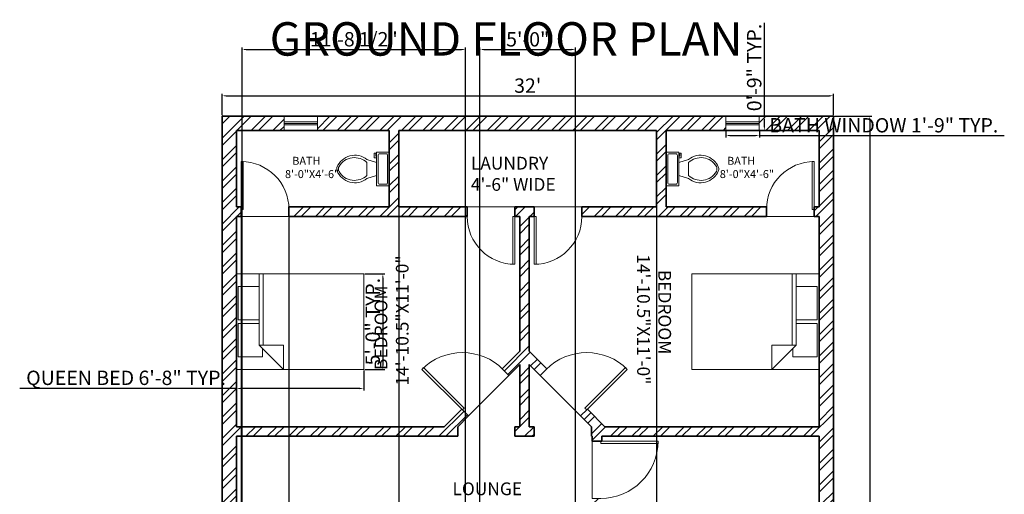
# Model space of a CAD drawing. Units: inches. Extents: x 287 to 905, y 1151 to 2037.
# Tile 5 of 5: x 287 to 905, y 1739 to 2037. Entities that reach past the tile are written whole.
import ezdxf

# ---------------------------------------------------------------- set-up
doc = ezdxf.new("R2010")
doc.units = ezdxf.units.IN
for name, color, linetype, lineweight in [('A-ANNO-DIMS', 2, 'Continuous', 18), ('A-ANNO-TEXT', 7, 'Continuous', 25), ('A-AREA-IDEN', 7, 'Continuous', 18), ('A-DOOR', 4, 'Continuous', 18), ('A-FLOR-FIXT', 8, 'Continuous', 18), ('A-FURN', 9, 'Continuous', 18), ('A-WALL', 7, 'Continuous', 35), ('A-WALL-PATT', 252, 'Continuous', 13)]:
    doc.layers.add(name, color=color, linetype=linetype, lineweight=lineweight)
doc.layers.add('A-GLAZ', color=244, linetype='Continuous', lineweight=18, true_color=0x991b1e)
doc.styles.get("Standard").update_dxf_attribs({"font": 'arial.ttf'})
doc.dimstyles.new('ISO-25', dxfattribs={"dimtxt": 9, "dimasz": 2.5, "dimexe": 1.25, "dimexo": 0.625, "dimtad": 1, "dimlunit": 3, "dimtxsty": 'Standard', "dimcen": 2.5, "dimadec": 0, "dimazin": 0, "dimtfac": 1, "dimtmove": 0, "dimatfit": 3, "dimfxl": 1, "dimarcsym": 0})

# ---------------------------------------------------------------- blocks, each defined once
blk = doc.blocks.new('*U3')
for p, q in [((0, 0), (0, -6)), ((-40, 0), (-40, -6))]:
    blk.add_line(p, q)
blk.add_lwpolyline([(0, 0), (0, 40), (-1.75, 40), (-1.75, 0)], close=True)
blk.add_arc((0, 0), 40, 90, 180)
blk = doc.blocks.new('*U2')
for p, q in [((0, 0), (0, -6)), ((40, 0), (40, -6))]:
    blk.add_line(p, q)
blk.add_lwpolyline([(0, 0), (0, 40), (1.75, 40), (1.75, 0)], close=True)
blk.add_arc((0, 0), 40, 0, 90)
blk = doc.blocks.new('*U5')
for p, q in [((-40, 0), (-40, 6)), ((0, 0), (0, 6))]:
    blk.add_line(p, q)
blk.add_lwpolyline([(0, 0), (0, -40), (-1.75, -40), (-1.75, 0)], close=True)
blk.add_arc((0, 0), 40, 180, 270)
blk = doc.blocks.new('*U4')
for p, q in [((0, 0), (0, 6)), ((40, 0), (40, 6))]:
    blk.add_line(p, q)
blk.add_lwpolyline([(0, 0), (0, -40), (1.75, -40), (1.75, 0)], close=True)
blk.add_arc((0, 0), 40, 270, 0)
blk = doc.blocks.new('*U6')
for p, q in [((0, 0), (0, -6)), ((40, 0), (40, -6))]:
    blk.add_line(p, q)
blk.add_lwpolyline([(0, 0), (0, 40), (1.75, 40), (1.75, 0)], close=True)
blk.add_arc((0, 0), 40, 0, 90)
blk = doc.blocks.new('Bed - Queen')
for p, q in [((0, -80.00003), (0, 0)), ((0, 0), (59.99999, 0)), ((59.99999, 0), (59.99999, -80.00003)), ((7.99999, -1.2), (28.79998, -1.2)), ((7.99999, -14.4), (7.99999, -1.2)), ((28.79998, -1.2), (28.79998, -14.4)), ((31.19999, -1.2), (51.99999, -1.2)), ((31.19999, -14.4), (31.19999, -1.2)), ((51.99999, -1.2), (51.99999, -16.4)), ((0, -14.4), (44.8, -14.4)), ((44.8, -16.8), (0, -16.8)), ((59.99999, -29.6), (44.8, -14.4)), ((44.8, -14.4), (44.8, -29.6)), ((51.99999, -16.4), (46.79936, -16.4)), ((44.8, -29.6), (59.99999, -29.6)), ((59.99999, -80.00003), (0, -80.00003))]:
    blk.add_line(p, q)
blk = doc.blocks.new('*U12')
for p, q in [((9.5, -6), (9.5, -2)), ((-10, -8.5), (-8, -8.5)), ((-10, -9.5), (-10, -8.5)), ((-7, -9.5), (-10, -9.5)), ((-8, -8.5), (-8, -8)), ((-7, -8), (-7, -9.5)), ((-4, -8), (-6, -14)), ((4, -8), (6, -14)), ((4, -14), (-4, -14))]:
    blk.add_line(p, q)
blk.add_lwpolyline([(10.5, -8), (10.5, 0), (-10.5, 0), (-10.5, -8)], close=True)
for points in [[(-9.5, -2), (-9.5, -6)], [(8.5, -1), (-8.5, -1)], [(-8.5, -7), (8.5, -7)]]:
    blk.add_lwpolyline(points)
for centre, radius, start, end in [((-8.62, -1.88), 0.884, 81.8699, 188.1301), ((-8.62, -6.12), 0.884, 171.8699, 278.1301), ((8.62, -1.88), 0.884, 351.8699, 98.1301), ((8.62, -6.12), 0.884, 261.8699, 8.1301), ((3.52, -21.58), 12.17, 141.46911, 247.97143), ((4.2, -21.82), 11.33, 136.36773, 238.94682), ((-3.52, -21.58), 12.17, 292.02843, 38.53071), ((-4.2, -21.82), 11.33, 301.05301, 43.63209), ((0, -27.88), 4, 245.73182, 294.26817), ((0, -29), 4, 254.86053, 285.13947)]:
    blk.add_arc(centre, radius, start, end)
blk = doc.blocks.new('*D13')
at = {"layer": 'A-ANNO-DIMS', "color": 0, "lineweight": -2, "transparency": 16777216}
for p, q in [((413.86, 1977.46), (413.86, 1990.88)), ((416.36, 1989.63), (795.36, 1989.63)), ((797.86, 1977.46), (797.86, 1990.88))]:
    blk.add_line(p, q, dxfattribs=at)
at = {"layer": 'A-ANNO-DIMS', "color": 0, "transparency": 16777216}
for points in [[(416.36, 1990.05), (416.36, 1989.22), (413.86, 1989.63)], [(795.36, 1990.05), (795.36, 1989.22), (797.86, 1989.63)]]:
    blk.add_solid(points, dxfattribs=at)
at = {"layer": 'Defpoints', "color": 0, "transparency": 16777216}
for p in [(797.86, 1989.63), (413.86, 1976.83), (797.86, 1976.83)]:
    blk.add_point(p, dxfattribs=at)
at = {"layer": 'A-ANNO-DIMS', "color": 0, "transparency": 16777216, "insert": (605.86, 1994.86), "char_height": 9, "attachment_point": 5}
blk.add_mtext("32'", dxfattribs=at)
blk = doc.blocks.new('*D14')
at = {"layer": 'A-ANNO-DIMS', "color": 0, "lineweight": -2, "transparency": 16777216}
for p, q in [((798.48, 1976.83), (822.01, 1976.83)), ((820.76, 1974.33), (820.76, 1280.33)), ((798.48, 1277.83), (822.01, 1277.83))]:
    blk.add_line(p, q, dxfattribs=at)
at = {"layer": 'A-ANNO-DIMS', "color": 0, "transparency": 16777216}
for points in [[(820.35, 1974.33), (821.18, 1974.33), (820.76, 1976.83)], [(820.35, 1280.33), (821.18, 1280.33), (820.76, 1277.83)]]:
    blk.add_solid(points, dxfattribs=at)
at = {"layer": 'Defpoints', "color": 0, "transparency": 16777216}
for p in [(797.86, 1976.83), (797.86, 1277.83), (820.76, 1277.83)]:
    blk.add_point(p, dxfattribs=at)
at = {"layer": 'A-ANNO-DIMS', "color": 0, "transparency": 16777216, "insert": (815.54, 1627.33), "char_height": 9, "attachment_point": 5, "rotation": 90}
blk.add_mtext('58\'-3"', dxfattribs=at)
blk = doc.blocks.new('WIN-21IN')
for p, q in [((-10.5, 1), (10.5, 1)), ((-10.5, 0), (10.5, 0)), ((-10.5, -1), (10.5, -1))]:
    blk.add_line(p, q)
blk.add_lwpolyline([(-10.5, 4.5), (10.5, 4.5), (10.5, -4.5), (-10.5, -4.5)], close=True)
blk = doc.blocks.new('*D18')
at = {"layer": 'A-ANNO-DIMS', "color": 0, "lineweight": -2, "transparency": 16777216}
for p, q in [((422.86, 1817.21), (422.86, 1804.58)), ((502.86, 1817.21), (502.86, 1804.58)), ((422.86, 1805.83), (286.72, 1805.83)), ((500.36, 1805.83), (425.36, 1805.83))]:
    blk.add_line(p, q, dxfattribs=at)
at = {"layer": 'A-ANNO-DIMS', "color": 0, "transparency": 16777216}
for points in [[(425.36, 1806.25), (425.36, 1805.42), (422.86, 1805.83)], [(500.36, 1806.25), (500.36, 1805.42), (502.86, 1805.83)]]:
    blk.add_solid(points, dxfattribs=at)
at = {"layer": 'Defpoints', "color": 0, "transparency": 16777216}
for p in [(422.86, 1817.83), (502.86, 1817.83), (422.86, 1805.83)]:
    blk.add_point(p, dxfattribs=at)
at = {"layer": 'A-ANNO-DIMS', "color": 0, "transparency": 16777216, "insert": (353.54, 1811.39), "char_height": 9, "attachment_point": 5}
blk.add_mtext('QUEEN BED 6\'-8" TYP.', dxfattribs=at)
blk = doc.blocks.new('*D19')
at = {"layer": 'A-ANNO-DIMS', "color": 0, "lineweight": -2, "transparency": 16777216}
for p, q in [((503.48, 1877.83), (516.11, 1877.83)), ((514.86, 1875.33), (514.86, 1820.33)), ((503.48, 1817.83), (516.11, 1817.83))]:
    blk.add_line(p, q, dxfattribs=at)
at = {"layer": 'A-ANNO-DIMS', "color": 0, "transparency": 16777216}
for points in [[(514.44, 1875.33), (515.27, 1875.33), (514.86, 1877.83)], [(514.44, 1820.33), (515.27, 1820.33), (514.86, 1817.83)]]:
    blk.add_solid(points, dxfattribs=at)
at = {"layer": 'Defpoints', "color": 0, "transparency": 16777216}
for p in [(502.86, 1877.83), (502.86, 1817.83), (514.86, 1817.83)]:
    blk.add_point(p, dxfattribs=at)
at = {"layer": 'A-ANNO-DIMS', "color": 0, "transparency": 16777216, "insert": (509.64, 1847.83), "char_height": 9, "attachment_point": 5, "rotation": 90}
blk.add_mtext('5\'-0" TYP.', dxfattribs=at)
blk = doc.blocks.new('*D20')
at = {"layer": 'A-ANNO-DIMS', "color": 0, "lineweight": -2, "transparency": 16777216}
for p, q in [((730.36, 1967.21), (730.36, 1963.43)), ((751.36, 1967.21), (751.36, 1963.43)), ((732.86, 1964.68), (748.86, 1964.68)), ((751.36, 1964.68), (905.25, 1964.68))]:
    blk.add_line(p, q, dxfattribs=at)
at = {"layer": 'A-ANNO-DIMS', "color": 0, "transparency": 16777216}
for points in [[(732.86, 1965.1), (732.86, 1964.27), (730.36, 1964.68)], [(748.86, 1965.1), (748.86, 1964.27), (751.36, 1964.68)]]:
    blk.add_solid(points, dxfattribs=at)
at = {"layer": 'Defpoints', "color": 0, "transparency": 16777216}
for p in [(730.36, 1967.83), (751.36, 1967.83), (751.36, 1964.68)]:
    blk.add_point(p, dxfattribs=at)
at = {"layer": 'A-ANNO-DIMS', "color": 0, "transparency": 16777216, "insert": (829.55, 1969.96), "char_height": 9, "attachment_point": 5}
blk.add_mtext('BATH WINDOW 1\'-9" TYP.', dxfattribs=at)
blk = doc.blocks.new('*D21')
at = {"layer": 'A-ANNO-DIMS', "color": 0, "lineweight": -2, "transparency": 16777216}
for p, q in [((754.51, 1976.83), (754.51, 2035.44)), ((751.98, 1976.83), (755.76, 1976.83)), ((754.51, 1970.33), (754.51, 1974.33)), ((751.98, 1967.83), (755.76, 1967.83))]:
    blk.add_line(p, q, dxfattribs=at)
at = {"layer": 'A-ANNO-DIMS', "color": 0, "transparency": 16777216}
for points in [[(754.09, 1974.33), (754.92, 1974.33), (754.51, 1976.83)], [(754.09, 1970.33), (754.92, 1970.33), (754.51, 1967.83)]]:
    blk.add_solid(points, dxfattribs=at)
at = {"layer": 'Defpoints', "color": 0, "transparency": 16777216}
for p in [(751.36, 1976.83), (754.51, 1976.83), (751.36, 1967.83)]:
    blk.add_point(p, dxfattribs=at)
at = {"layer": 'A-ANNO-DIMS', "color": 0, "transparency": 16777216, "insert": (749.29, 2007.39), "char_height": 9, "attachment_point": 5, "rotation": 90}
blk.add_mtext('0\'-9" TYP.', dxfattribs=at)
blk = doc.blocks.new('*D32')
at = {"layer": 'A-ANNO-DIMS', "color": 0, "lineweight": -2, "transparency": 16777216}
for p, q in [((426.39, 1284.46), (426.39, 2019.96)), ((428.89, 2018.71), (564.36, 2018.71)), ((566.86, 1284.46), (566.86, 2019.96))]:
    blk.add_line(p, q, dxfattribs=at)
at = {"layer": 'A-ANNO-DIMS', "color": 0, "transparency": 16777216}
for points in [[(428.89, 2019.12), (428.89, 2018.29), (426.39, 2018.71)], [(564.36, 2019.12), (564.36, 2018.29), (566.86, 2018.71)]]:
    blk.add_solid(points, dxfattribs=at)
at = {"layer": 'Defpoints', "color": 0, "transparency": 16777216}
for p in [(566.86, 2018.71), (426.39, 1283.83), (566.86, 1283.83)]:
    blk.add_point(p, dxfattribs=at)
at = {"layer": 'A-ANNO-DIMS', "color": 0, "transparency": 16777216, "insert": (496.62, 2023.99), "char_height": 9, "attachment_point": 5}
blk.add_mtext('11\'-8 1/2"', dxfattribs=at)
blk = doc.blocks.new('*D33')
at = {"layer": 'A-ANNO-DIMS', "color": 0, "lineweight": -2, "transparency": 16777216}
for p, q in [((575.86, 1284.46), (575.86, 2019.96)), ((578.36, 2018.71), (633.36, 2018.71)), ((635.86, 1284.46), (635.86, 2019.96))]:
    blk.add_line(p, q, dxfattribs=at)
at = {"layer": 'A-ANNO-DIMS', "color": 0, "transparency": 16777216}
for points in [[(578.36, 2019.12), (578.36, 2018.29), (575.86, 2018.71)], [(633.36, 2019.12), (633.36, 2018.29), (635.86, 2018.71)]]:
    blk.add_solid(points, dxfattribs=at)
at = {"layer": 'Defpoints', "color": 0, "transparency": 16777216}
for p in [(635.86, 2018.71), (575.86, 1283.83), (635.86, 1283.83)]:
    blk.add_point(p, dxfattribs=at)
at = {"layer": 'A-ANNO-DIMS', "color": 0, "transparency": 16777216, "insert": (605.86, 2023.93), "char_height": 9, "attachment_point": 5}
blk.add_mtext('5\'-0"', dxfattribs=at)
blk = doc.blocks.new('*D37')
at = {"layer": 'A-ANNO-DIMS', "color": 0, "lineweight": -2, "transparency": 16777216}
for p, q in [((524.86, 1967.21), (524.86, 1157.65)), ((686.86, 1967.21), (686.86, 1157.65)), ((527.36, 1158.9), (684.36, 1158.9))]:
    blk.add_line(p, q, dxfattribs=at)
at = {"layer": 'A-ANNO-DIMS', "color": 0, "transparency": 16777216}
for points in [[(527.36, 1159.32), (527.36, 1158.49), (524.86, 1158.9)], [(684.36, 1159.32), (684.36, 1158.49), (686.86, 1158.9)]]:
    blk.add_solid(points, dxfattribs=at)
at = {"layer": 'Defpoints', "color": 0, "transparency": 16777216}
for p in [(524.86, 1967.83), (686.86, 1967.83), (686.86, 1158.9)]:
    blk.add_point(p, dxfattribs=at)
at = {"layer": 'A-ANNO-DIMS', "color": 0, "transparency": 16777216, "insert": (605.86, 1164.13), "char_height": 9, "attachment_point": 5}
blk.add_mtext('13\'-6"', dxfattribs=at)
blk = doc.blocks.new('*D38')
at = {"layer": 'A-ANNO-DIMS', "color": 0, "lineweight": -2, "transparency": 16777216}
for p, q in [((425.86, 1913.21), (425.86, 1157.65)), ((455.86, 1913.21), (455.86, 1157.65)), ((428.36, 1158.9), (453.36, 1158.9))]:
    blk.add_line(p, q, dxfattribs=at)
at = {"layer": 'A-ANNO-DIMS', "color": 0, "transparency": 16777216}
for points in [[(428.36, 1159.32), (428.36, 1158.49), (425.86, 1158.9)], [(453.36, 1159.32), (453.36, 1158.49), (455.86, 1158.9)]]:
    blk.add_solid(points, dxfattribs=at)
at = {"layer": 'Defpoints', "color": 0, "transparency": 16777216}
for p in [(425.86, 1913.83), (455.86, 1913.83), (455.86, 1158.9)]:
    blk.add_point(p, dxfattribs=at)
at = {"layer": 'A-ANNO-DIMS', "color": 0, "transparency": 16777216, "insert": (440.86, 1164.12), "char_height": 9, "attachment_point": 5}
blk.add_mtext('2\'-6"', dxfattribs=at)

msp = doc.modelspace()

# ---------------------------------------------------------------- hatches: boundary and pattern name
at = {"layer": 'A-WALL-PATT'}
h = msp.add_hatch(dxfattribs=at)
h.set_pattern_fill('ANSI32', color=256)
h.paths.add_polyline_path([(422.857, 1775.833), (561.857, 1775.833), (561.857, 1781.833), (568.629, 1788.605), (564.387, 1792.848), (553.372, 1781.833), (422.857, 1781.833), (422.857, 1913.833), (425.857, 1913.833), (425.857, 1919.833), (422.857, 1919.833), (422.857, 1967.833), (452.78, 1967.833), (452.78, 1976.833), (413.857, 1976.833), (413.857, 1502.833), (436.063, 1502.833), (436.063, 1511.833), (422.857, 1511.833), (422.857, 1625.833), (474.857, 1625.833), (474.857, 1631.833), (422.857, 1631.833)])
h = msp.add_hatch(dxfattribs=at)
h.set_pattern_fill('ANSI32', color=256)
h.paths.add_polyline_path([(604.357, 1511.833), (519.857, 1511.833), (519.857, 1625.833), (607.357, 1625.833), (607.357, 1631.833), (510.857, 1631.833), (510.857, 1625.833), (513.857, 1625.833), (513.857, 1511.833), (496.063, 1511.833), (496.063, 1502.833), (604.357, 1502.833)])
h.paths.add_polyline_path([(652.357, 1511.833), (652.357, 1514.833), (643.357, 1514.833), (643.357, 1511.833), (640.357, 1511.833), (640.357, 1505.833), (643.357, 1505.833), (643.357, 1370.833), (690.607, 1370.833), (690.607, 1379.833), (652.357, 1379.833)])
h.paths.add_polyline_path([(797.857, 1582.055), (788.857, 1582.055), (788.857, 1571.833), (703.357, 1571.833), (703.357, 1574.833), (697.357, 1574.833), (697.357, 1571.833), (652.357, 1571.833), (652.357, 1574.833), (646.357, 1574.833), (646.357, 1562.833), (652.357, 1562.833), (652.357, 1565.833), (788.857, 1565.833), (788.857, 1379.833), (750.607, 1379.833), (750.607, 1370.833), (797.857, 1370.833)])
h.paths.add_polyline_path([(797.857, 1673.833), (788.857, 1673.833), (788.857, 1631.833), (685.357, 1631.833), (685.357, 1625.833), (697.357, 1625.833), (697.357, 1604.833), (703.357, 1604.833), (703.357, 1625.833), (788.857, 1625.833), (788.857, 1603.055), (797.857, 1603.055)])
h.paths.add_polyline_path([(797.857, 1976.833), (751.357, 1976.833), (751.357, 1967.833), (788.857, 1967.833), (788.857, 1919.833), (785.857, 1919.833), (785.857, 1913.833), (788.857, 1913.833), (788.857, 1781.833), (654.342, 1781.833), (643.328, 1792.848), (639.085, 1788.605), (645.857, 1781.833), (645.857, 1775.833), (646.357, 1775.833), (646.357, 1772.833), (652.357, 1772.833), (652.357, 1775.833), (788.857, 1775.833), (788.857, 1733.833), (797.857, 1733.833)])
h.paths.add_polyline_path([(755.857, 1919.833), (692.857, 1919.833), (692.857, 1967.833), (730.357, 1967.833), (730.357, 1976.833), (473.78, 1976.833), (473.78, 1967.833), (518.857, 1967.833), (518.857, 1919.833), (455.857, 1919.833), (455.857, 1913.833), (567.857, 1913.833), (567.857, 1919.833), (524.857, 1919.833), (524.857, 1967.833), (686.857, 1967.833), (686.857, 1919.833), (639.857, 1919.833), (639.857, 1913.833), (755.857, 1913.833)])
h.paths.add_polyline_path([(606.857, 1913.833), (609.857, 1913.833), (609.857, 1919.833), (597.857, 1919.833), (597.857, 1913.833), (600.857, 1913.833), (600.857, 1829.319), (589.842, 1818.304), (594.085, 1814.061), (600.857, 1820.833), (600.857, 1781.833), (597.857, 1781.833), (597.857, 1775.833), (609.857, 1775.833), (609.857, 1781.833), (606.857, 1781.833), (606.857, 1820.833), (613.629, 1814.061), (617.872, 1818.304), (606.857, 1829.319)])
h.paths.add_polyline_path([(652.357, 1736.833), (646.357, 1736.833), (646.357, 1631.833), (643.357, 1631.833), (643.357, 1625.833), (646.357, 1625.833), (646.357, 1604.833), (652.357, 1604.833), (652.357, 1625.833), (655.357, 1625.833), (655.357, 1631.833), (652.357, 1631.833)])

# ---------------------------------------------------------------- linework, layer by layer
at = {"layer": 'A-DOOR'}
for p, q in [((567.857, 1919.833), (597.857, 1919.833)), ((609.857, 1919.833), (639.857, 1919.833)), ((425.857, 1913.833), (455.857, 1913.833)), ((785.857, 1913.833), (755.857, 1913.833)), ((594.085, 1814.061), (568.629, 1788.605)), ((613.629, 1814.061), (639.085, 1788.605)), ((646.357, 1772.833), (646.357, 1736.833))]:
    msp.add_line(p, q, dxfattribs=at)
at = {"layer": 'A-WALL'}
for p, q in [((413.857, 1976.833), (797.857, 1976.833)), ((413.857, 1976.833), (413.857, 1277.833)), ((797.857, 1976.833), (797.857, 1277.833)), ((422.857, 1967.833), (518.857, 1967.833)), ((422.857, 1967.833), (422.857, 1919.833)), ((518.857, 1967.833), (518.857, 1919.833)), ((524.857, 1967.833), (524.857, 1919.833)), ((524.857, 1967.833), (686.857, 1967.833)), ((686.857, 1967.833), (686.857, 1919.833)), ((692.857, 1967.833), (692.857, 1919.833)), ((692.857, 1967.833), (788.857, 1967.833)), ((788.857, 1967.833), (788.857, 1919.833)), ((422.857, 1919.833), (425.857, 1919.833)), ((425.857, 1913.833), (425.857, 1919.833)), ((455.857, 1913.833), (455.857, 1919.833)), ((455.857, 1919.833), (518.857, 1919.833)), ((524.857, 1919.833), (567.857, 1919.833)), ((567.857, 1913.833), (567.857, 1919.833)), ((597.857, 1913.833), (597.857, 1919.833)), ((597.857, 1919.833), (609.857, 1919.833)), ((609.857, 1913.833), (609.857, 1919.833)), ((639.857, 1913.833), (639.857, 1919.833)), ((639.857, 1919.833), (686.857, 1919.833)), ((692.857, 1919.833), (755.857, 1919.833)), ((755.857, 1913.833), (755.857, 1919.833)), ((785.857, 1913.833), (785.857, 1919.833)), ((785.857, 1919.833), (788.857, 1919.833)), ((422.857, 1913.833), (425.857, 1913.833)), ((422.857, 1913.833), (422.857, 1781.833)), ((455.857, 1913.833), (567.857, 1913.833)), ((597.857, 1913.833), (600.857, 1913.833)), ((600.857, 1913.833), (600.857, 1829.319)), ((606.857, 1913.833), (606.857, 1829.319)), ((606.857, 1913.833), (609.857, 1913.833)), ((639.857, 1913.833), (755.857, 1913.833)), ((785.857, 1913.833), (788.857, 1913.833)), ((788.857, 1913.833), (788.857, 1781.833)), ((600.857, 1829.319), (589.842, 1818.304)), ((606.857, 1829.319), (617.872, 1818.304)), ((600.857, 1820.833), (594.085, 1814.061)), ((600.857, 1820.833), (600.857, 1781.833)), ((606.857, 1820.833), (613.629, 1814.061)), ((606.857, 1820.833), (606.857, 1781.833)), ((589.842, 1818.304), (594.085, 1814.061)), ((617.872, 1818.304), (613.629, 1814.061)), ((564.387, 1792.848), (553.372, 1781.833)), ((568.629, 1788.605), (561.857, 1781.833)), ((564.387, 1792.848), (568.629, 1788.605)), ((643.328, 1792.848), (639.085, 1788.605)), ((639.085, 1788.605), (645.857, 1781.833)), ((643.328, 1792.848), (654.342, 1781.833)), ((422.857, 1781.833), (553.372, 1781.833)), ((561.857, 1781.833), (561.857, 1775.833)), ((597.857, 1781.833), (597.857, 1775.833)), ((597.857, 1781.833), (600.857, 1781.833)), ((606.857, 1781.833), (609.857, 1781.833)), ((609.857, 1781.833), (609.857, 1775.833)), ((645.857, 1781.833), (645.857, 1775.833)), ((654.342, 1781.833), (788.857, 1781.833)), ((422.857, 1775.833), (561.857, 1775.833)), ((422.857, 1775.833), (422.857, 1631.833)), ((597.857, 1775.833), (609.857, 1775.833)), ((645.857, 1775.833), (646.357, 1775.833)), ((646.357, 1775.833), (646.357, 1772.833)), ((652.357, 1775.833), (652.357, 1772.833)), ((652.357, 1775.833), (788.857, 1775.833)), ((788.857, 1775.833), (788.857, 1631.833)), ((646.357, 1772.833), (652.357, 1772.833))]:
    msp.add_line(p, q, dxfattribs=at)

# ---------------------------------------------------------------- block references
at = {"layer": 'A-DOOR', "xscale": 0.7500000000000029, "yscale": 0.7500000000000029, "zscale": 0.7500000000000029}
for name, p in [('*U2', (425.857, 1918.333)), ('*U3', (785.857, 1918.333)), ('*U5', (597.857, 1913.833)), ('*U4', (609.857, 1913.833))]:
    msp.add_blockref(name, p, dxfattribs=at)
at = {"layer": 'A-DOOR'}
for name, p, xscale, yscale, zscale, rotation in [('*U2', (564.811, 1792.424), 0.9000000000000019, 0.9000000000000019, 0.9000000000000019, 45.00000000000039), ('*U2', (642.903, 1792.424), -0.9000000000000019, 0.9000000000000019, 0.9000000000000019, 315.0000000000018), ('*U6', (651.757, 1772.833), 0.9000000000001479, 0.9000000000001479, 0.9000000000001479, 270)]:
    msp.add_blockref(name, p, dxfattribs=dict(at, xscale=xscale, yscale=yscale, zscale=zscale, rotation=rotation))
at = {"layer": 'A-FLOR-FIXT', "rotation": 270}
msp.add_blockref('*U12', (518.857, 1943.674), dxfattribs=at)
at = {"layer": 'A-FLOR-FIXT', "xscale": -1, "rotation": 90}
msp.add_blockref('*U12', (692.857, 1943.674), dxfattribs=at)
at = {"layer": 'A-FURN', "xscale": -1, "rotation": 89.99999999999952}
msp.add_blockref('Bed - Queen', (422.857, 1877.833), dxfattribs=at)
at = {"layer": 'A-FURN', "rotation": 269.9999999999996}
msp.add_blockref('Bed - Queen', (788.857, 1877.833), dxfattribs=at)
at = {"layer": 'A-GLAZ'}
for p in [(463.28, 1972.333), (740.857, 1972.333)]:
    msp.add_blockref('WIN-21IN', p, dxfattribs=at)

# ---------------------------------------------------------------- texts
at = {"layer": 'A-ANNO-TEXT', "insert": (443.757, 2035.84), "char_height": 21, "attachment_point": 1}
msp.add_mtext_dynamic_manual_height_columns('GROUND FLOOR PLAN', width=345.82434, gutter_width=12.5, heights=[0], dxfattribs=at)
at = {"layer": 'A-AREA-IDEN', "attachment_point": 1}
for s, width, insert, char_height in [('   BATH\\P8\'-0"X4\'-6"', 32.58174, (453.378, 1951.312), 5), ('LAUNDRY 4\'-6" WIDE', 56.90459, (570.134, 1951.312), 8), ('   BATH\\P8\'-0"X4\'-6"', 32.58174, (726.525, 1951.312), 5), ('  LOUNGE\\P18\'-4.5"X12\'-0"', 72.39263, (553.702, 1746.891), 8)]:
    msp.add_mtext_dynamic_manual_height_columns(s, width=width, gutter_width=12.5, heights=[0], dxfattribs=dict(at, insert=insert, char_height=char_height))
at = {"layer": 'A-AREA-IDEN', "char_height": 8, "attachment_point": 1}
for insert, rotation in [((509.675, 1807.703), 90), ((695.923, 1890.154), 270)]:
    msp.add_mtext_dynamic_manual_height_columns('    BEDROOM\\P14\'-10.5"X11\'-0"', width=80.50627, gutter_width=12.5, heights=[0], dxfattribs=dict(at, insert=insert, rotation=rotation))

# ---------------------------------------------------------------- dimensions: what is measured, and where the dimension line sits
at = {"layer": 'A-ANNO-DIMS'}
for base, p1, p2, override, picture, middle in [((566.857, 2018.708), (426.388, 1283.833), (566.857, 1283.833), {"dimdec": 1, "dimlfac": 1, "dimrnd": 0, "dimzin": 1, "dimdsep": 46, "dimlunit": 4, "dimfrac": 2}, '*D32', (496.622, 2023.987)), ((635.857, 2018.708), (575.857, 1283.833), (635.857, 1283.833), {"dimdec": 1, "dimlfac": 1, "dimrnd": 0, "dimzin": 1, "dimdsep": 46, "dimlunit": 4, "dimfrac": 2}, '*D33', (605.857, 2023.928)), ((797.857, 1989.633), (413.857, 1976.833), (797.857, 1976.833), {"dimclrd": 0, "dimclre": 0, "dimclrt": 0}, '*D13', (605.857, 1994.856)), ((686.857, 1158.902), (524.857, 1967.833), (686.857, 1967.833), {"dimdec": 1, "dimlfac": 1, "dimrnd": 0, "dimzin": 1, "dimdsep": 46, "dimlunit": 4, "dimfrac": 2}, '*D37', (605.857, 1164.125)), ((455.857, 1158.902), (425.857, 1913.833), (455.857, 1913.833), {"dimdec": 1, "dimlfac": 1, "dimrnd": 0, "dimzin": 1, "dimdsep": 46, "dimlunit": 4, "dimfrac": 2}, '*D38', (440.857, 1164.122))]:
    dim = msp.add_linear_dim(base=base, p1=p1, p2=p2, dimstyle='ISO-25', override=override, dxfattribs=at)
    dim.commit()
    dim.dimension.update_dxf_attribs({"geometry": picture, "text_midpoint": middle})
for base, p1, p2, angle, text, picture, middle in [((754.507, 1976.833), (751.357, 1967.833), (751.357, 1976.833), 90, '<> TYP.', '*D21', (749.287, 2007.388)), ((514.857, 1817.833), (502.857, 1877.833), (502.857, 1817.833), 270, '<> TYP.', '*D19', (509.637, 1847.833)), ((422.857, 1805.833), (502.857, 1817.833), (422.857, 1817.833), 180, 'QUEEN BED <> TYP.', '*D18', (353.537, 1811.388))]:
    dim = msp.add_linear_dim(base=base, p1=p1, p2=p2, angle=angle, text=text, dimstyle='ISO-25', override={"dimdec": 1, "dimlfac": 1, "dimrnd": 0, "dimzin": 1, "dimdsep": 46, "dimlunit": 4, "dimfrac": 2}, dxfattribs=at)
    dim.commit()
    dim.dimension.update_dxf_attribs({"geometry": picture, "text_midpoint": middle})
dim = msp.add_linear_dim(base=(751.357, 1964.683), p1=(730.357, 1967.833), p2=(751.357, 1967.833), text='BATH WINDOW <> TYP.', dimstyle='ISO-25', override={"dimdec": 1, "dimlfac": 1, "dimrnd": 0, "dimzin": 1, "dimdsep": 46, "dimlunit": 4, "dimfrac": 2}, dxfattribs=at)
dim.commit()
dim.dimension.update_dxf_attribs({"geometry": '*D20', "text_midpoint": (829.555, 1969.965)})
dim = msp.add_linear_dim(base=(820.762, 1277.833), p1=(797.857, 1976.833), p2=(797.857, 1277.833), angle=90, dimstyle='ISO-25', override={"dimclrd": 0, "dimclre": 0, "dimclrt": 0}, dxfattribs=at)
dim.commit()
dim.dimension.update_dxf_attribs({"geometry": '*D14', "text_midpoint": (815.538, 1627.333)})

doc.saveas('drawing.dxf')
